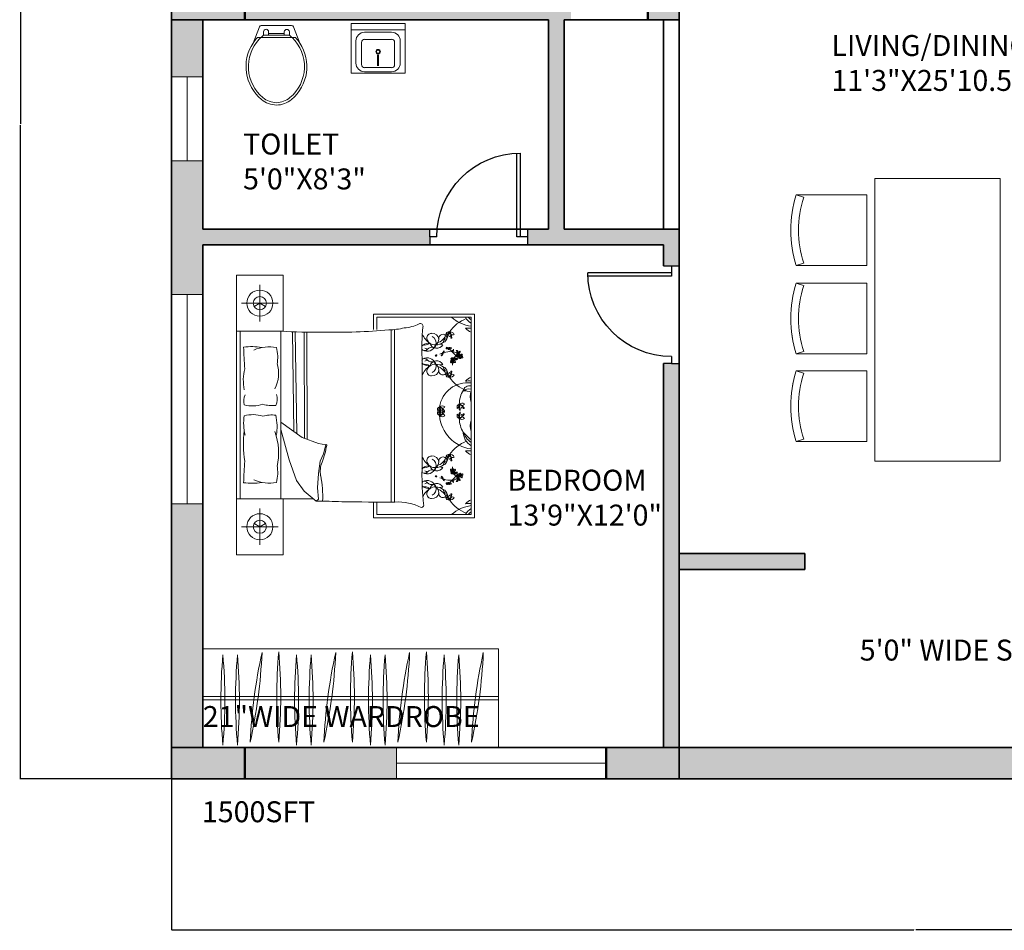
# Model space of a CAD drawing. Units: inches. Extents: x -28 to 485, y -861 to 54.
# Tile 1 of 14: x -28 to 254, y -861 to -600. Entities that reach past the tile are written whole.
import ezdxf

# ---------------------------------------------------------------- set-up
doc = ezdxf.new("R2010")
doc.units = ezdxf.units.IN
doc.header["$MEASUREMENT"] = 0
for name, color, linetype, lineweight in [('A-ANNO-DIMS', 2, 'Continuous', 18), ('A-ANNO-TEXT', 7, 'Continuous', 18), ('A-AREA-IDEN', 7, 'Continuous', 18), ('A-COLS', 7, 'Continuous', 50), ('A-COLS-PATT', 8, 'Continuous', 13), ('A-DOOR', 3, 'Continuous', 25), ('A-FLOR-CASE', 8, 'Continuous', 18), ('A-FLOR-FIXT', 9, 'Continuous', 18), ('A-FURN', 8, 'Continuous', 13), ('A-GLAZ', 4, 'Continuous', 18), ('A-WALL', 7, 'Continuous', 35), ('A-WALL-PATT', 34, 'Continuous', 13)]:
    doc.layers.add(name, color=color, linetype=linetype, lineweight=lineweight)
doc.styles.get("Standard").update_dxf_attribs({"font": 'arial.ttf'})
doc.dimstyles.get("Standard").update_dxf_attribs({"dimtxt": 0.18, "dimasz": 0.18, "dimexe": 0.18, "dimexo": 0.0625, "dimgap": 0.09, "dimtad": 0, "dimtih": 1, "dimtoh": 1, "dimdec": 0, "dimzin": 0, "dimdsep": 46, "dimlunit": 3, "dimtxsty": 'Standard', "dimcen": 0.09, "dimadec": 0, "dimazin": 0, "dimtfac": 1, "dimtdec": 0, "dimtofl": 0, "dimtmove": 0, "dimatfit": 3, "dimfxl": 1, "dimtolj": 1, "dimtzin": 0, "dimarcsym": 0})

# ---------------------------------------------------------------- blocks, each defined once
blk = doc.blocks.new('М14 600х655')
for p, q in [((-655, 600), (-655, 0)), ((-655, 600), (-655, 0)), ((-655, 0), (-655, 600)), ((0, 600), (-655, 600)), ((0, 0), (0, 600)), ((0, 525), (-655, 525)), ((-165, 494), (-490, 494)), ((-596, 388), (-596, 121)), ((-528, 370), (-528, 103)), ((-165, 408), (-490, 408)), ((-127, 103), (-127, 370)), ((-59, 121), (-59, 388)), ((-334, 87), (-334, 220)), ((-321, 87), (-321, 220)), ((-655, 0), (-655, 0)), ((-655, 0), (-655, 0)), ((-655, 0), (0, 0)), ((-655, 0), (0, 0)), ((-490, 65), (-165, 65)), ((-490, 15), (-165, 15))]:
    blk.add_line(p, q)
for radius in [27.6, 19.3]:
    blk.add_circle((-327, 259), radius)
for centre, radius, start, end in [((-490, 388), 106, 90, 180), ((-165, 388), 106, 0, 90), ((-490, 370), 38.2, 90, 180), ((-165, 370), 38.2, 0, 90), ((-490, 121), 106, 180, 270), ((-165, 121), 106, 270, 0), ((-490, 103), 38.2, 180, 270), ((-165, 103), 38.2, 270, 0)]:
    blk.add_arc(centre, radius, start, end)
blk = doc.blocks.new('BED-DOUBLE-WITH-NIGHTSTANDS')
for p, q in [((0, 0), (0, 80.08)), ((6.67, 66.84), (6.67, 77.31)), ((11.91, 72.08), (1.44, 72.08)), ((39.26, 64.51), (39.26, 68.96)), ((39.26, 68.96), (68.11, 68.96)), ((40.19, 68.03), (40.19, 64.5)), ((67.18, 68.03), (40.19, 68.03)), ((67.18, 11.5), (67.18, 68.03)), ((68.11, 68.96), (68.11, 10.57)), ((1.03, 64.07), (1.03, 16.02)), ((12.66, 16.02), (12.66, 64.07)), ((15.98, 63.85), (16.38, 35.34)), ((16.8, 63.82), (17.22, 34.74)), ((19.33, 63.78), (19.45, 33.37)), ((20.15, 63.78), (20.27, 33.06)), ((44.25, 64.43), (44.25, 15.09)), ((45.25, 64.51), (45.25, 15.09)), ((59.06, 60.14), (58.15, 60.31)), ((53.12, 56.3), (53.12, 23.78)), ((59.06, 54.54), (58.15, 54.36)), ((12.66, 38.02), (18.76, 33.63)), ((15.04, 27.14), (12.66, 35.87)), ((18.76, 33.63), (23.47, 31.84)), ((23.47, 31.84), (25.57, 31.52)), ((25.57, 31.52), (24.92, 28.93)), ((24.92, 28.93), (23.95, 26.82)), ((17.14, 21.3), (15.04, 27.14)), ((23.95, 26.82), (23.47, 23.25)), ((23.47, 23.25), (23.14, 19.19)), ((59.06, 24.99), (58.15, 25.16)), ((19.41, 18.22), (17.14, 21.3)), ((22.82, 15.3), (19.41, 18.22)), ((23.14, 19.19), (23.47, 15.95)), ((59.06, 19.39), (58.15, 19.21)), ((0, 16.02), (21.98, 16.02)), ((23.47, 15.95), (22.82, 15.3)), ((39.26, 10.57), (39.26, 15.1)), ((40.19, 15.1), (40.19, 11.5)), ((6.67, 13.24), (6.67, 2.78)), ((40.19, 11.5), (67.18, 11.5)), ((68.11, 10.57), (39.26, 10.57)), ((11.91, 8.01), (1.44, 8.01))]:
    blk.add_line(p, q)
for points in [[(0, 64.07), (13.35, 64.07), (13.35, 80.08), (0, 80.08)], [(6.67, 72.08), (5.06, 71.14)], [(6.67, 72.08), (8.29, 71.14)], [(13.35, 16.02), (13.35, 0), (0, 0)], [(6.67, 8.01), (5.06, 8.94)], [(6.67, 8.01), (8.29, 8.94)]]:
    blk.add_lwpolyline(points)
for points in [[(43.62, 64.41, 0.056112), (48.03, 64.99, 0.095341), (52.27, 66.12)], [(2, 59.47, -0.074897), (7.23, 59.37, 0.472817)], [(7.52, 43.09, -0.14099), (2.18, 42.93, -0.235245)], [(7.52, 39.67, 0.14099), (2.18, 39.83, 0.235245)], [(2, 20.62, 0.074897), (7.23, 20.71, -0.472817)], [(30.15, 15.13, 0.001242), (45.35, 15.09, -0.127202), (52.92, 13.49)]]:
    blk.add_lwpolyline(points, format="xyb")
for centre, radius in [((6.67, 72.08), 3.74), ((6.67, 72.08), 1.87), ((64.11, 56.84), 0.204), ((61.96, 55.51), 0.204), ((61.96, 24.02), 0.204), ((64.11, 22.68), 0.204), ((6.67, 8.01), 3.74), ((6.67, 8.01), 1.87)]:
    blk.add_circle(centre, radius)
for centre, radius, start, end in [((68.59, 75.81), 10.46, 228.1144, 262.255), ((69.99, 70.57), 5.1, 209.8884, 236.5383), ((70.94, 72.4), 6.35, 223.5186, 233.6964), ((52.68, 65.51), 0.73, 336.5219, 123.8264), ((131.01, 58.75), 77.93, 175.2402, 181.8035), ((69.62, 57.92), 10.46, 111.4092, 145.6135), ((68.81, 67.71), 4.25, 221.0454, 247.4453), ((66.52, 79.36), 14.47, 266.3481, 272.5919), ((22.44, 207.63), 143.9, 266.1, 270.9282), ((27.68, 251.44), 187.71, 269.1145, 274.8735), ((58.76, 65.61), 6.06, 203.6453, 236.3329), ((55.85, 62.08), 1.35, 88.9462, 185.5144), ((56.04, 61.53), 1.91, 7.1143, 95.0551), ((55.32, 60.77), 1.86, 338.5779, 68.4181), ((56.48, 64.35), 3.78, 288.2955, 328.7386), ((59.12, 61.97), 1.2, 19.1312, 189.736), ((58.76, 62.26), 1.5, 285.6955, 4.031), ((60.43, 62.21), 0.737, 126.7319, 206.0245), ((60.79, 62.99), 0.867, 76.272, 177.0484), ((59.47, 64.76), 1.79, 284.7031, 328.6173), ((61.96, 62.49), 1.65, 125.7657, 194.5347), ((53.85, 65.41), 7.32, 332.8176, 347.4827), ((61.24, 62.69), 1.16, 20.9613, 102.2885), ((61.86, 63.85), 0.873, 181.7131, 301.5367), ((59, 62.09), 2.64, 2.0648, 41.1598), ((60.59, 63.07), 0.856, 316.2238, 62.3173), ((61.09, 62.57), 0.0682, 20.2667, 316.2271), ((61.51, 62.18), 0.13, 168.5166, 2.0648), ((61.45, 62.19), 0.0631, 52.0591, 168.5166), ((-760.15, 15.33), 763.42, 2.85022, 3.31479), ((9.33, 49.26), 10.32, 78.2417, 114.8684), ((1.06, 56.61), 10.73, 348.9631, 14.8961), ((54, 59.28), 0.964, 127.675, 162.5814), ((53.71, 63.39), 3.32, 259.249, 301.1782), ((54.57, 60.82), 2.55, 240.8249, 340.7178), ((55.15, 57.49), 3.09, 85.2696, 124.215), ((56.85, 62.5), 2.41, 193.079, 274.7067), ((55.94, 57.8), 1.64, 74.8529, 138.4347), ((57.33, 61.13), 1.99, 196.8663, 330.0915), ((56.5, 59.87), 0.497, 254.8529, 12.6959), ((55.15, 57.49), 3.09, 53.6555, 57.2989), ((55.62, 61.86), 2.33, 305.9599, 357.6409), ((56.78, 64.39), 4.3, 273.4924, 303.7117), ((60.76, 60.64), 1.6, 128.4175, 173.8338), ((60.19, 59.12), 0.158, 125.0752, 284.7644), ((60.43, 59.18), 0.34, 127.3642, 168.4363), ((60.17, 59.45), 0.49, 277.4968, 341.2737), ((60.56, 59.22), 0.195, 88.1325, 178.8919), ((60.95, 59.02), 0.422, 136.3462, 189.6513), ((60.75, 59.46), 0.204, 183.2768, 356.7232), ((61.39, 59.1), 0.668, 164.2829, 186.9148), ((60.6, 59.09), 0.334, 312.3208, 40.2111), ((61.31, 59.47), 0.474, 201.6382, 274.947), ((60.68, 58.82), 0.619, 42.3896, 66.5724), ((61.13, 59.18), 0.337, 10.9597, 52.2379), ((61.33, 59.15), 0.156, 274.947, 37.5263), ((54, 59.28), 0.964, 196.6343, 225.5483), ((53.81, 59.69), 1.2, 246.1646, 318.4347), ((55.03, 61.2), 2.3, 240.0851, 262.564), ((57.16, 57.12), 0.251, 169.5864, 349.5616), ((57.25, 57.11), 0.154, 349.5616, 167.2949), ((61.28, 51.56), 6.63, 110.1059, 116.9968), ((59.06, 57.02), 0.42, 129.5056, 182.6421), ((57.85, 58), 1.27, 308.4388, 328.836), ((57.63, 59.02), 2.26, 296.5064, 305.3102), ((57.61, 57.86), 1.29, 336.3901, 344.4871), ((59.01, 57.53), 0.163, 83.9457, 185.6216), ((58.36, 57.69), 0.671, 328.836, 0.8141), ((58.71, 57.49), 0.384, 306.5232, 32.4668), ((59.16, 57.79), 0.163, 112.5583, 214.2343), ((59.06, 58.08), 0.384, 265.7131, 351.6568), ((58.72, 58.29), 0.671, 297.3659, 329.344), ((58.21, 58.87), 1.29, 313.6929, 321.7899), ((59.64, 57.99), 0.42, 115.5379, 168.6744), ((58.21, 58.6), 1.27, 329.344, 349.7412), ((61.28, 51.56), 6.63, 86.1723, 106.4158), ((57.2, 58.31), 2.26, 352.8698, 1.6736), ((60.71, 58.98), 0.176, 189.6513, 312.3208), ((66.93, 63.72), 7.6, 217.9541, 226.8459), ((61.66, 57.07), 0.93, 253.6301, 325.4631), ((61.92, 55.78), 0.658, 82.0748, 142.6895), ((61.86, 58.27), 0.163, 112.5583, 214.2343), ((61.75, 58.56), 0.384, 265.7131, 351.6568), ((61.42, 58.77), 0.671, 297.3659, 329.344), ((61.45, 54.86), 3.33, 60.7959, 85.244), ((54.37, 50.07), 10.94, 37.8256, 47.7588), ((60.91, 59.35), 1.29, 313.6929, 321.7899), ((61.87, 56.57), 0.565, 273.8774, 357.1501), ((62.33, 58.47), 0.42, 115.5379, 168.6744), ((60.9, 59.07), 1.27, 329.344, 349.7412), ((62.09, 56.97), 0.547, 262.0748, 308.2393), ((59.89, 58.78), 2.26, 352.8698, 1.6736), ((62.87, 56.86), 0.547, 215.1128, 261.2773), ((63.31, 56.83), 0.93, 197.889, 269.722), ((65.87, 54.52), 3.99, 130.182, 149.456), ((63.07, 58.33), 0.228, 33.0979, 123.1364), ((58.05, 55.12), 5.96, 31.1156, 34.8118), ((62.74, 57.94), 0.617, 2.3172, 70.5201), ((63.67, 56.79), 0.658, 139.3812, 199.9959), ((62.44, 57.27), 0.93, 310.9365, 22.7695), ((62.87, 57.22), 0.675, 285.6484, 332.2957), ((63.25, 57.78), 0.178, 135.7354, 318.1297), ((62.95, 58.07), 0.236, 315.7354, 31.1156), ((62.75, 57.57), 0.547, 319.3812, 5.5456), ((63.38, 57.79), 0.178, 68.2452, 250.6395), ((62.97, 58), 0.531, 352.6008, 57.1845), ((64.87, 54.44), 3.55, 111.7087, 116.2181), ((61.45, 54.86), 3.33, 47.5083, 55.9967), ((63.48, 58.12), 0.531, 252.8042, 349.6943), ((62.97, 57.17), 0.565, 331.1838, 51.6792), ((63.55, 56.5), 0.158, 125.0752, 284.7644), ((63.53, 58.17), 0.236, 248.2452, 323.6254), ((63.8, 56.56), 0.34, 93.635, 168.4363), ((63.33, 58.31), 0.617, 291.7087, 3.0299), ((63.75, 57.1), 0.2, 138.2946, 276.2474), ((63.53, 56.83), 0.49, 277.4968, 341.2737), ((63.83, 57.07), 0.278, 358.5719, 143.8954), ((58.93, 61.56), 5.96, 323.6254, 327.3216), ((63.92, 56.61), 0.195, 88.1325, 178.8919), ((63.99, 57.29), 0.281, 208.8493, 269.9355), ((63.75, 57.22), 0.321, 274.2123, 318.1587), ((64.31, 56.4), 0.422, 136.3462, 189.6513), ((63.81, 58.16), 0.228, 325.6077, 55.6462), ((64.75, 56.48), 0.668, 164.2829, 186.9148), ((64.73, 56.9), 0.643, 121.9501, 165.2442), ((63.96, 56.47), 0.334, 312.3208, 40.2111), ((64.67, 56.85), 0.474, 201.6382, 274.947), ((64.28, 57.14), 0.135, 262.868, 7.094), ((64.04, 56.2), 0.619, 42.3896, 66.5724), ((64.27, 57.26), 0.403, 278.5614, 22.5914), ((64.49, 56.56), 0.337, 10.9597, 118.7804), ((64.49, 57.27), 0.202, 44.3732, 121.9501), ((64.7, 56.53), 0.156, 274.947, 37.5263), ((1.85, 51.98), 10.19, 333.8761, 16.1746), ((54, 55.39), 0.964, 134.4517, 156.7144), ((54, 55.39), 0.964, 203.2856, 232.325), ((53.71, 51.28), 3.32, 58.8218, 100.2867), ((58.76, 49.06), 6.06, 123.6671, 158.5059), ((54.57, 53.85), 2.55, 19.2822, 119.1751), ((53.81, 54.99), 1.2, 41.5653, 113.8354), ((55.15, 57.18), 3.09, 235.785, 274.7304), ((55.03, 53.47), 2.3, 97.436, 119.9149), ((56.85, 52.18), 2.41, 85.2933, 166.921), ((55.94, 56.87), 1.64, 221.5653, 285.1471), ((57.33, 53.55), 1.99, 29.9085, 163.1337), ((55.32, 53.9), 1.86, 291.5819, 21.4221), ((56.5, 54.81), 0.497, 347.3041, 105.1471), ((55.15, 57.18), 3.09, 302.7011, 306.3445), ((55.62, 52.81), 2.33, 2.3591, 54.0401), ((56.78, 50.29), 4.3, 56.2883, 86.5076), ((56.48, 50.32), 3.78, 31.2614, 71.7045), ((60.76, 54.03), 1.6, 186.1662, 231.5825), ((58.76, 52.42), 1.5, 355.969, 74.3045), ((61.4, 55.17), 0.158, 125.0752, 284.7644), ((61.65, 55.23), 0.34, 93.635, 168.4363), ((61.85, 56.68), 0.675, 228.342, 274.9894), ((61.6, 55.76), 0.2, 138.2946, 276.2474), ((61.38, 55.5), 0.49, 277.4968, 341.2737), ((61.68, 55.73), 0.278, 358.5719, 143.8954), ((61.77, 55.27), 0.195, 88.1325, 178.8919), ((61.84, 55.95), 0.281, 208.8493, 269.9355), ((61.6, 55.89), 0.321, 274.2123, 318.1587), ((62.16, 55.06), 0.422, 136.3462, 189.6513), ((61.92, 55.02), 0.176, 189.6513, 312.3208), ((65.87, 54.52), 3.99, 175.2415, 182.8929), ((62.6, 55.14), 0.668, 164.2829, 186.9148), ((62.58, 55.56), 0.643, 121.9501, 165.2442), ((61.81, 55.14), 0.334, 312.3208, 40.2111), ((62.52, 55.52), 0.474, 201.6382, 274.947), ((62.13, 55.81), 0.135, 262.868, 7.094), ((61.89, 54.87), 0.619, 42.3896, 66.5724), ((62.12, 55.92), 0.403, 278.5614, 22.5914), ((62.34, 55.23), 0.337, 10.9597, 118.7804), ((65.87, 54.52), 3.99, 156.1523, 156.9499), ((62.34, 55.94), 0.202, 44.3732, 121.9501), ((62.97, 56.41), 0.565, 181.4625, 249.4747), ((62.55, 55.2), 0.156, 274.947, 37.5263), ((63.02, 56.51), 0.675, 248.3627, 295.0101), ((62.69, 55.67), 0.658, 20.6625, 81.2773), ((64.07, 56.36), 0.176, 189.6513, 312.3208), ((16.01, 49.96), 14.08, 166.3427, 191.1841), ((55.85, 52.59), 1.35, 174.4856, 271.0538), ((56.04, 53.15), 1.91, 264.9449, 352.8857), ((59.12, 52.71), 1.2, 170.264, 340.8688), ((60.43, 52.46), 0.737, 153.9755, 233.2681), ((60.79, 51.69), 0.867, 182.9516, 283.728), ((59.47, 49.92), 1.79, 31.3827, 75.2969), ((61.96, 52.19), 1.65, 165.4653, 234.2343), ((53.85, 49.26), 7.32, 12.5173, 27.1824), ((59, 52.59), 2.64, 318.8402, 357.9352), ((60.59, 51.6), 0.856, 297.6827, 43.7762), ((61.86, 50.82), 0.873, 58.4633, 178.2869), ((61.24, 51.98), 1.16, 257.7115, 339.0387), ((69.62, 56.75), 10.46, 214.3865, 248.5908), ((61.13, 52.12), 0.113, 43.7762, 339.7183), ((61.51, 52.5), 0.13, 357.9352, 191.4834), ((61.45, 52.48), 0.0631, 191.4834, 307.9409), ((68.81, 46.96), 4.25, 112.5547, 138.9546), ((66.17, 41.19), 8.09, 82.8636, 171.8197), ((66.74, 46.53), 1.88, 76.3898, 169.0739), ((66.52, 35.31), 14.47, 87.4081, 93.6519), ((5.99, 44.03), 3.96, 153.3437, 196.1026), ((7.37, 44.56), 4.25, 335.0183, 18.5407), ((74.19, 42.33), 10.46, 152.5854, 175.5377), ((66.48, 45.12), 2.37, 72.8609, 131.9049), ((65.43, 42.24), 4.68, 68.117, 96.6195), ((72.68, 45.26), 5.75, 162.9798, 196.4569), ((10.2, 52.53), 9.81, 254.1707, 275.9871), ((58.4, 41.51), 0.867, 106.1963, 206.9726), ((56.38, 42.39), 1.79, 314.6273, 358.5415), ((59.67, 41.66), 1.65, 155.6899, 224.4589), ((58.94, 41.49), 1.16, 50.8855, 132.2127), ((58.91, 42.8), 0.873, 211.6373, 331.4609), ((58.2, 41.49), 0.856, 346.148, 92.2415), ((57.3, 39.84), 2.64, 31.989, 71.0841), ((51.18, 40.16), 7.32, 2.7418, 17.407), ((64.01, 42.31), 0.867, 106.1963, 206.9726), ((61.98, 43.19), 1.79, 314.6273, 358.5415), ((65.27, 42.46), 1.65, 155.6899, 224.4589), ((64.54, 42.29), 1.16, 50.8855, 132.2127), ((64.51, 43.6), 0.873, 211.6373, 331.4609), ((63.8, 42.29), 0.856, 346.148, 92.2415), ((62.91, 40.64), 2.64, 31.989, 71.0841), ((56.78, 40.96), 7.32, 2.7418, 17.407), ((75.64, 42.98), 8.5, 174.3643, 175.6213), ((81.47, 38.5), 15.2, 160.0972, 160.2783), ((16.3, 37.72), 14.27, 171.5249, 193.96), ((10.2, 30.23), 9.81, 84.0129, 105.8293), ((-2.51, 36.66), 14.12, 349.8617, 13.6238), ((58.4, 40.68), 0.867, 153.0274, 253.8037), ((56.38, 39.81), 1.79, 1.4585, 45.3727), ((59.67, 40.53), 1.65, 135.5411, 204.3101), ((51.18, 42.04), 7.32, 342.593, 357.2582), ((57.3, 42.35), 2.64, 288.9159, 328.011), ((58.2, 40.71), 0.856, 267.7585, 13.852), ((58.91, 39.39), 0.873, 28.5391, 148.3627), ((58.94, 40.71), 1.16, 227.7873, 309.1145), ((68.59, 40.66), 10.46, 184.4623, 262.255), ((58.87, 41.3), 0.0682, 50.1909, 346.0209), ((58.92, 40.88), 0.113, 13.852, 309.9245), ((59.44, 41.17), 0.13, 198.4408, 31.989), ((59.37, 41.15), 0.0631, 81.9833, 198.4408), ((59.44, 41.02), 0.13, 328.011, 161.5592), ((59.37, 41.04), 0.0631, 161.5592, 278.0167), ((64.01, 39.88), 0.867, 153.0274, 253.8037), ((61.98, 39.01), 1.79, 1.4585, 45.3727), ((65.27, 39.73), 1.65, 135.5411, 204.3101), ((56.78, 41.24), 7.32, 342.593, 357.2582), ((62.91, 41.55), 2.64, 288.9159, 328.011), ((63.8, 39.91), 0.856, 267.7585, 13.852), ((64.52, 40.08), 0.113, 13.852, 309.9245), ((64.47, 42.1), 0.0682, 50.1909, 346.0209), ((64.98, 41.95), 0.0631, 81.9833, 198.4408), ((64.98, 40.24), 0.0631, 161.5592, 278.0167), ((65.04, 41.98), 0.13, 198.4408, 31.989), ((65.04, 40.22), 0.13, 328.011, 161.5592), ((64.51, 38.59), 0.873, 28.5391, 148.3627), ((64.54, 39.91), 1.16, 227.7873, 309.1145), ((74.19, 39.86), 10.46, 184.4623, 207.4146), ((72.68, 36.94), 5.75, 163.5431, 197.0202), ((75.64, 39.22), 8.5, 184.3787, 185.6357), ((81.47, 43.7), 15.2, 199.7217, 199.9028), ((30.98, 31.59), 29.04, 172.2196, 189.497), ((-6.57, 29.12), 18.61, 348.0397, 19.2615), ((69.99, 35.42), 5.1, 181.272, 236.5383), ((72.72, 40.59), 9.45, 214.0123, 234.053), ((70.94, 37.25), 6.35, 197.8504, 233.6964), ((-4.69, 37.08), 31.06, 340.1194, 349.3383), ((25.64, 31.34), 0.193, 358.8623, 109.7536), ((69.62, 22.77), 10.46, 111.4092, 145.6135), ((58.76, 30.46), 6.06, 201.4941, 236.3329), ((55.85, 26.93), 1.35, 88.9462, 185.5144), ((56.04, 26.38), 1.91, 7.1143, 95.0551), ((60.79, 27.84), 0.867, 76.272, 177.0484), ((59.47, 29.61), 1.79, 284.7031, 328.6173), ((61.96, 27.34), 1.65, 125.7657, 194.5347), ((53.85, 30.27), 7.32, 332.8176, 347.4827), ((61.24, 27.55), 1.16, 20.9613, 102.2885), ((60.59, 27.92), 0.856, 316.2238, 62.3173), ((59, 26.94), 2.64, 2.0648, 41.1598), ((61.86, 28.71), 0.873, 181.7131, 301.5367), ((66.52, 44.21), 14.47, 266.3481, 272.5919), ((68.81, 32.56), 4.25, 221.0454, 247.4453), ((-760.15, 64.76), 763.42, 356.68521, 357.14978), ((1.06, 23.47), 10.73, 345.1039, 11.0369), ((30.48, 23.89), 6.52, 156.2616, 191.3392), ((53.71, 28.24), 3.32, 259.7133, 301.1782), ((55.15, 22.34), 3.09, 85.2696, 124.215), ((56.85, 27.35), 2.41, 193.079, 274.7067), ((57.33, 25.98), 1.99, 196.8663, 330.0915), ((55.32, 25.63), 1.86, 338.5779, 68.4181), ((55.62, 26.71), 2.33, 305.9599, 357.6409), ((56.78, 29.24), 4.3, 273.4924, 303.7117), ((56.48, 29.2), 3.78, 288.2955, 328.7386), ((59.12, 26.82), 1.2, 19.1312, 189.736), ((58.76, 27.11), 1.5, 285.6955, 4.031), ((60.76, 25.49), 1.6, 128.4175, 173.8338), ((60.43, 27.07), 0.737, 126.7319, 206.0245), ((61.09, 27.42), 0.0682, 20.2667, 316.2271), ((61.51, 27.03), 0.13, 168.5166, 2.0648), ((61.45, 27.04), 0.0631, 52.0591, 168.5166), ((-5.54, 16.67), 30.23, 357.4519, 11.3392), ((136.48, 22.83), 83.37, 179.3433, 185.6887), ((54, 24.13), 0.964, 127.675, 156.7144), ((54, 24.13), 0.964, 203.229, 225.5483), ((54.57, 25.67), 2.55, 240.8249, 340.7178), ((53.81, 24.54), 1.2, 246.1646, 318.4347), ((55.03, 26.06), 2.3, 240.0851, 262.564), ((55.94, 22.65), 1.64, 74.8529, 138.4347), ((56.5, 24.72), 0.497, 254.8529, 12.6959), ((55.15, 22.34), 3.09, 53.6555, 57.2989), ((57.16, 22.4), 0.251, 10.4384, 190.4136), ((61.4, 24.36), 0.158, 75.2356, 234.9248), ((61.65, 24.3), 0.34, 191.5637, 266.365), ((61.6, 23.76), 0.2, 83.7526, 221.7054), ((61.85, 22.84), 0.675, 85.0106, 131.658), ((61.66, 22.46), 0.93, 34.5369, 106.3699), ((61.92, 23.75), 0.658, 217.3105, 277.9252), ((61.38, 24.03), 0.49, 18.7263, 82.5032), ((61.68, 23.79), 0.278, 216.1046, 1.4281), ((61.77, 24.25), 0.195, 181.1081, 271.8675), ((61.84, 23.57), 0.281, 90.0645, 151.1507), ((61.6, 23.64), 0.321, 41.8413, 85.7877), ((54.37, 29.45), 10.94, 312.2412, 322.1744), ((61.92, 24.5), 0.176, 47.6792, 170.3487), ((62.16, 24.46), 0.422, 170.3487, 223.6538), ((65.87, 25.01), 3.99, 177.1071, 184.7585), ((61.87, 22.95), 0.565, 2.8499, 86.1226), ((62.6, 24.38), 0.668, 173.0852, 195.7171), ((62.58, 23.96), 0.643, 194.7558, 238.0499), ((62.09, 22.55), 0.547, 51.7607, 97.9252), ((61.81, 24.39), 0.334, 319.7889, 47.6792), ((62.52, 24.01), 0.474, 85.053, 158.3618), ((62.13, 23.71), 0.135, 352.906, 97.132), ((61.89, 24.66), 0.619, 293.4276, 317.6104), ((62.34, 24.29), 0.337, 241.2196, 349.0403), ((62.12, 23.6), 0.403, 337.4086, 81.4386), ((65.87, 25.01), 3.99, 203.0501, 203.8477), ((62.34, 23.59), 0.202, 238.0499, 315.6268), ((62.97, 23.11), 0.565, 110.5253, 178.5375), ((63.31, 22.7), 0.93, 90.278, 162.111), ((62.87, 22.67), 0.547, 98.7227, 144.8872), ((65.87, 25.01), 3.99, 210.544, 229.818), ((62.55, 24.33), 0.156, 322.4737, 85.053), ((63.02, 23.01), 0.675, 64.9899, 111.6373), ((62.69, 23.86), 0.658, 278.7227, 339.3375), ((63.67, 22.74), 0.658, 160.0041, 220.6188), ((62.44, 22.26), 0.93, 337.2305, 49.0635), ((62.87, 22.31), 0.675, 27.7043, 74.3516), ((62.97, 22.35), 0.565, 308.3208, 28.8162), ((63.55, 23.03), 0.158, 75.2356, 234.9248), ((63.8, 22.96), 0.34, 191.5637, 266.365), ((63.75, 22.43), 0.2, 83.7526, 221.7054), ((63.53, 22.69), 0.49, 18.7263, 82.5032), ((63.92, 22.92), 0.195, 181.1081, 271.8675), ((63.75, 22.31), 0.321, 41.8413, 85.7877), ((64.07, 23.17), 0.176, 47.6792, 170.3487), ((64.31, 23.13), 0.422, 170.3487, 223.6538), ((64.75, 23.05), 0.668, 173.0852, 195.7171), ((63.96, 23.05), 0.334, 319.7889, 47.6792), ((64.67, 22.68), 0.474, 85.053, 158.3618), ((64.04, 23.32), 0.619, 293.4276, 317.6104), ((64.49, 22.96), 0.337, 241.2196, 349.0403), ((64.27, 22.27), 0.403, 337.4086, 81.4386), ((64.7, 22.99), 0.156, 322.4737, 85.053), ((9.33, 30.82), 10.32, 245.1316, 281.7583), ((54, 20.25), 0.964, 134.4517, 153.558), ((54, 20.25), 0.964, 210.0293, 232.325), ((54.57, 18.71), 2.55, 19.2822, 119.1751), ((53.81, 19.84), 1.2, 41.5653, 113.8354), ((55.03, 18.32), 2.3, 97.436, 119.9149), ((55.94, 21.72), 1.64, 221.5653, 285.1471), ((57.33, 18.4), 1.99, 29.9085, 163.1337), ((56.5, 19.66), 0.497, 347.3041, 105.1471), ((57.25, 22.42), 0.154, 192.7051, 10.4384), ((61.28, 27.97), 6.63, 243.0032, 249.8941), ((57.85, 21.53), 1.27, 31.164, 51.5612), ((59.06, 22.5), 0.42, 177.3579, 230.4944), ((57.63, 20.5), 2.26, 54.6898, 63.4936), ((57.61, 21.66), 1.29, 15.5129, 23.6099), ((59.01, 21.99), 0.163, 174.3784, 276.0543), ((58.71, 22.03), 0.384, 327.5332, 53.4768), ((58.36, 21.84), 0.671, 359.1859, 31.164), ((59.16, 21.74), 0.163, 145.7657, 247.4417), ((59.06, 21.45), 0.384, 8.3432, 94.2869), ((58.72, 21.23), 0.671, 30.656, 62.6341), ((58.21, 20.66), 1.29, 38.2101, 46.3071), ((59.64, 21.53), 0.42, 191.3256, 244.4621), ((58.21, 20.93), 1.27, 10.2588, 30.656), ((61.28, 27.97), 6.63, 253.5842, 273.8277), ((57.2, 21.22), 2.26, 358.3264, 7.1302), ((60.19, 20.41), 0.158, 75.2356, 234.9248), ((60.43, 20.35), 0.34, 191.5637, 232.6358), ((60.17, 20.07), 0.49, 18.7263, 82.5032), ((60.56, 20.3), 0.195, 181.1081, 271.8675), ((60.71, 20.55), 0.176, 47.6792, 170.3487), ((60.95, 20.51), 0.422, 170.3487, 223.6538), ((60.75, 20.06), 0.204, 3.2768, 176.7232), ((61.39, 20.43), 0.668, 173.0852, 195.7171), ((60.6, 20.43), 0.334, 319.7889, 47.6792), ((61.31, 20.06), 0.474, 85.053, 158.3618), ((60.68, 20.7), 0.619, 293.4276, 317.6104), ((66.93, 15.8), 7.6, 133.1541, 142.0459), ((61.13, 20.34), 0.337, 307.7621, 349.0403), ((61.33, 20.37), 0.156, 322.4737, 85.053), ((61.86, 21.26), 0.163, 145.7657, 247.4417), ((61.45, 24.67), 3.33, 274.756, 299.2041), ((61.75, 20.97), 0.384, 8.3432, 94.2869), ((61.42, 20.76), 0.671, 30.656, 62.6341), ((60.91, 20.18), 1.29, 38.2101, 46.3071), ((62.33, 21.06), 0.42, 191.3256, 244.4621), ((60.9, 20.45), 1.27, 10.2588, 30.656), ((59.89, 20.74), 2.26, 358.3264, 7.1302), ((62.74, 21.59), 0.617, 289.4799, 357.6828), ((58.05, 24.41), 5.96, 325.1882, 328.8844), ((63.07, 21.2), 0.228, 236.8636, 326.9021), ((63.25, 21.74), 0.178, 41.8703, 224.2646), ((62.95, 21.45), 0.236, 328.8844, 44.2646), ((62.75, 21.95), 0.547, 354.4544, 40.6188), ((63.38, 21.74), 0.178, 109.3605, 291.7548), ((62.97, 21.52), 0.531, 302.8155, 7.3992), ((64.87, 25.09), 3.55, 243.7819, 248.2913), ((61.45, 24.67), 3.33, 304.0033, 312.4917), ((63.48, 21.4), 0.531, 10.3057, 107.1958), ((63.53, 21.36), 0.236, 36.3746, 111.7548), ((63.33, 21.21), 0.617, 356.9701, 68.2913), ((63.83, 22.46), 0.278, 216.1046, 1.4281), ((58.93, 17.96), 5.96, 32.6784, 36.3746), ((63.99, 22.24), 0.281, 90.0645, 151.1507), ((63.81, 21.37), 0.228, 304.3538, 34.3923), ((64.73, 22.63), 0.643, 194.7558, 238.0499), ((64.28, 22.38), 0.135, 352.906, 97.132), ((64.49, 22.25), 0.202, 238.0499, 315.6268), ((53.71, 16.14), 3.32, 58.8218, 99.1554), ((58.76, 13.91), 6.06, 123.6671, 153.2997), ((55.15, 22.04), 3.09, 235.785, 274.7304), ((56.85, 17.03), 2.41, 85.2933, 166.921), ((55.85, 17.44), 1.35, 174.4856, 271.0538), ((56.04, 18), 1.91, 264.9449, 352.8857), ((55.32, 18.75), 1.86, 291.5819, 21.4221), ((55.15, 22.04), 3.09, 302.7011, 306.3445), ((55.62, 17.67), 2.33, 2.3591, 54.0401), ((56.78, 15.14), 4.3, 56.2883, 86.5076), ((56.48, 15.18), 3.78, 31.2614, 71.7045), ((59.12, 17.56), 1.2, 170.264, 340.8688), ((58.76, 17.27), 1.5, 355.969, 74.3045), ((60.76, 18.89), 1.6, 186.1662, 231.5825), ((60.43, 17.31), 0.737, 153.9755, 233.2681), ((61.96, 17.04), 1.65, 165.4653, 234.2343), ((53.85, 14.11), 7.32, 12.5173, 27.1824), ((59, 17.44), 2.64, 318.8402, 357.9352), ((60.59, 16.46), 0.856, 297.6827, 43.7762), ((61.13, 16.97), 0.113, 43.7762, 339.7183), ((61.51, 17.35), 0.13, 357.9352, 191.4834), ((61.45, 17.33), 0.0631, 191.4834, 307.9409), ((24.81, -58.13), 73.46, 85.8294, 91.553), ((52.87, 14.23), 0.739, 273.98, 27.3412), ((59.47, 14.77), 1.79, 31.3827, 75.2969), ((60.79, 16.54), 0.867, 182.9516, 283.728), ((61.86, 15.67), 0.873, 58.4633, 178.2869), ((61.24, 16.83), 1.16, 257.7115, 339.0387), ((69.62, 21.6), 10.46, 214.3865, 248.5908), ((68.81, 11.81), 4.25, 112.5547, 138.9546), ((66.52, 0.17), 14.47, 87.4081, 93.6519), ((68.59, 3.71), 10.46, 97.745, 131.8856), ((69.99, 8.96), 5.1, 123.4617, 150.1116), ((70.94, 7.13), 6.35, 126.3036, 136.4814)]:
    blk.add_arc(centre, radius, start, end)
blk = doc.blocks.new('WARDROBE-HANGING')
for p, q in [((84.7, 28.23), (0, 28.23)), ((0, 28.23), (0, 0)), ((84.7, 28.23), (84.7, 0)), ((84.7, 14.59), (0, 14.59)), ((84.7, 13.65), (0, 13.65)), ((84.7, 0), (0, 0))]:
    blk.add_line(p, q)
for centre, start, end in [((153.74, 13.55), 175.0028, 184.9972), ((-142.25, 13.55), 355.0028, 4.9972), ((157.93, 13.55), 175.0028, 184.9972), ((-138.07, 13.55), 355.0028, 4.9972), ((-131.46, 33.65), 347.508, 357.5023), ((162.01, -4.96), 167.508, 177.5023), ((169.76, 14.46), 175.0028, 184.9972), ((-126.23, 14.46), 355.0028, 4.9972), ((174.85, 13.55), 175.0028, 184.9972), ((-121.15, 13.55), 355.0028, 4.9972), ((179.03, 13.55), 175.0028, 184.9972), ((-116.97, 13.55), 355.0028, 4.9972), ((-110.36, 33.65), 347.508, 357.5023), ((183.11, -4.96), 167.508, 177.5023), ((190.86, 14.46), 175.0028, 184.9972), ((-105.13, 14.46), 355.0028, 4.9972), ((196.03, 13.55), 175.0028, 184.9972), ((-99.97, 13.55), 355.0028, 4.9972), ((200.21, 13.55), 175.0028, 184.9972), ((-95.78, 13.55), 355.0028, 4.9972), ((204.29, -4.96), 167.508, 177.5023), ((-89.17, 33.65), 347.508, 357.5023), ((212.05, 14.46), 175.0028, 184.9972), ((-83.95, 14.46), 355.0028, 4.9972), ((217.13, 13.55), 175.0028, 184.9972), ((-78.86, 13.55), 355.0028, 4.9972), ((221.31, 13.55), 175.0028, 184.9972), ((-74.68, 13.55), 355.0028, 4.9972), ((225.4, -4.96), 167.508, 177.5023), ((-68.07, 33.65), 347.508, 357.5023)]:
    blk.add_arc(centre, 148.56, start, end)
blk = doc.blocks.new('WC-FLOOR-MOUNTED')
for p, q in [((3.27, 19.35), (4.23, 19.35)), ((4.23, 19.35), (8.71, 19.35)), ((13.2, 19.35), (8.71, 19.35)), ((13.2, 19.35), (14.16, 19.35))]:
    blk.add_line(p, q)
for points in [[(8.71, 22.81), (4.36, 22.81, 0.31031), (3.82, 22.44), (2.03, 17.79, 0.209071)], [(8.71, 22.81), (13.07, 22.81, -0.31031), (13.6, 22.44), (15.39, 17.79, -0.209071)], [(5.01, 20.04, 0.022712), (4.23, 19.35, 0.162618)], [(5.01, 20.04), (5.01, 21, -1), (6.47, 21), (6.47, 20.5)], [(8.71, 20.04), (5.01, 20.04, 0.022712)], [(8.71, 20.04), (12.41, 20.04, -0.476108)], [(12.41, 20.04), (12.41, 21, 1), (10.96, 21), (10.96, 20.5)], [(12.41, 20.04, -0.022712), (13.2, 19.35, -0.162618)], [(2.03, 17.79, 0.383919), (4.43, 1.64, 0.163732), (8.71, 0, 0.359733)], [(3.77, 18.89, 0.431639), (4.86, 2.17, 0.162618), (8.71, 0.68, 0.470877)], [(3.27, 19.35, 0.040937), (2.03, 17.79, 0.163732)], [(4.23, 19.35, 0.014165), (3.77, 18.89, 0.162618)], [(13.2, 19.35, -0.448546), (12.57, 2.17, -0.162618), (8.71, 0.68, -0.470877)], [(15.39, 17.79, -0.383919), (13, 1.64, -0.163732), (8.71, 0, -0.359733)], [(14.16, 19.35, -0.040937), (15.39, 17.79, -0.163732)]]:
    blk.add_lwpolyline(points, format="xyb")
for points in [[(10.96, 20.5), (6.47, 20.5)], [(6.47, 20.5), (6.47, 20.04)], [(10.96, 20.5), (10.96, 20.04)]]:
    blk.add_lwpolyline(points)
blk = doc.blocks.new('CHAIR-DINING')
for p, q in [((20.22, 20.23), (18.08, 19.55)), ((20.22, 0), (18.08, 0.68))]:
    blk.add_line(p, q)
blk.add_lwpolyline([(20.23, 0), (0, 0), (0, 20.23), (20.23, 20.23, -0.153703), (20.23, 0)], format="xyb")
for radius in [33.37, 31.13]:
    blk.add_arc((-11.59, 10.12), radius, 342.3544, 17.6456)
blk = doc.blocks.new('TABLE-DINING-RECT')
blk.add_lwpolyline([(0, 80.93), (35.97, 80.93), (35.97, 0), (0, 0)], close=True)
blk = doc.blocks.new('DOOR-SWING-24')
for p, q in [((2, 2.25), (2, 26.25)), ((3, 2.25), (3, 26.25)), ((0, 4.5), (0, 0)), ((28, 2.25), (28, 4.5)), ((0, 2.25), (2, 2.25)), ((2, 2.25), (3, 2.25)), ((26, 2.25), (28, 2.25)), ((28, 2.25), (28, 0))]:
    blk.add_line(p, q)
blk.add_arc((2, 2.25), 24, 0, 90)
blk = doc.blocks.new('WINDOW-60IN')
for p, q in [((0, 60), (0, 0)), ((9, 60), (0, 60)), ((4.5, 60), (4.5, 0)), ((9, 0), (9, 60)), ((0, 0), (9, 0))]:
    blk.add_line(p, q)
blk = doc.blocks.new('WINDOW-24IN')
for p, q in [((0, 24), (0, 0)), ((9, 24), (0, 24)), ((4.5, 24), (4.5, 0)), ((9, 0), (9, 24)), ((9, 0), (0, 0))]:
    blk.add_line(p, q)
blk = doc.blocks.new('*D52')
at = {"layer": 'A-ANNO-DIMS', "color": 0, "lineweight": -2, "transparency": 16777216}
for p, q in [((15.28, -817.93), (15.28, -861.3)), ((441.28, -817.93), (441.28, -861.3)), ((15.46, -861.12), (227.99, -861.12)), ((441.1, -861.12), (228.58, -861.12))]:
    blk.add_line(p, q, dxfattribs=at)
at = {"layer": 'A-ANNO-DIMS', "color": 0, "transparency": 16777216}
for points in [[(15.46, -861.09), (15.46, -861.15), (15.28, -861.12)], [(441.1, -861.09), (441.1, -861.15), (441.28, -861.12)]]:
    blk.add_solid(points, dxfattribs=at)
at = {"layer": 'Defpoints', "color": 0, "transparency": 16777216}
for p in [(15.28, -817.87), (441.28, -817.87), (441.28, -861.12)]:
    blk.add_point(p, dxfattribs=at)
at = {"layer": 'A-ANNO-DIMS', "color": 0, "transparency": 16777216, "insert": (228.28, -861.12), "char_height": 0.18, "attachment_point": 5}
blk.add_mtext('\\A1;426', dxfattribs=at)
blk = doc.blocks.new('*D56')
at = {"layer": 'A-ANNO-DIMS', "color": 0, "lineweight": -2, "transparency": 16777216}
for p, q in [((15.22, -442.87), (-28.15, -442.87)), ((-27.97, -443.05), (-27.97, -630.18)), ((-27.97, -817.69), (-27.97, -630.55)), ((15.22, -817.87), (-28.15, -817.87))]:
    blk.add_line(p, q, dxfattribs=at)
at = {"layer": 'A-ANNO-DIMS', "color": 0, "transparency": 16777216}
for points in [[(-28, -443.05), (-27.94, -443.05), (-27.97, -442.87)], [(-28, -817.69), (-27.94, -817.69), (-27.97, -817.87)]]:
    blk.add_solid(points, dxfattribs=at)
at = {"layer": 'Defpoints', "color": 0, "transparency": 16777216}
for p in [(15.28, -442.87), (-27.97, -817.87), (15.28, -817.87)]:
    blk.add_point(p, dxfattribs=at)
at = {"layer": 'A-ANNO-DIMS', "color": 0, "transparency": 16777216, "insert": (-27.97, -630.37), "char_height": 0.18, "attachment_point": 5}
blk.add_mtext('\\A1;375', dxfattribs=at)

msp = doc.modelspace()

# ---------------------------------------------------------------- hatches: boundary and pattern name
at = {"layer": 'A-COLS-PATT'}
h = msp.add_hatch(color=256, dxfattribs=at)
h.dxf.hatch_style = 1
h.paths.add_polyline_path([(441.285, -591.367), (420.285, -591.367), (420.285, -595.867), (420.285, -600.367), (441.285, -600.367)])
h.paths.add_polyline_path([(304.691, -588.367), (295.785, -588.367), (295.785, -600.367), (304.691, -600.367)])
h.paths.add_polyline_path([(160.785, -588.367), (151.785, -588.367), (151.785, -600.367), (160.785, -600.367)])
h.paths.add_polyline_path([(36.285, -591.367), (24.285, -591.367), (15.285, -591.367), (15.285, -600.367), (36.285, -600.367)])
h.paths.add_polyline_path([(36.285, -808.867), (15.285, -808.867), (15.285, -817.867), (36.285, -817.867)])
h.paths.add_polyline_path([(160.785, -808.867), (139.785, -808.867), (139.785, -817.867), (160.785, -817.867)])
h.paths.add_polyline_path([(316.785, -808.867), (295.785, -808.867), (295.785, -817.867), (316.785, -817.867)])
h.paths.add_polyline_path([(441.285, -808.867), (420.285, -808.867), (420.285, -817.867), (441.285, -817.867)])
h.paths.add_polyline_path([(36.285, -442.867), (15.285, -442.867), (15.285, -451.867), (36.285, -451.867)])
h.paths.add_polyline_path([(160.785, -442.867), (139.785, -442.867), (139.785, -451.867), (160.785, -451.867)])
h.paths.add_polyline_path([(316.785, -442.867), (295.785, -442.867), (295.785, -451.867), (316.785, -451.867)])
h.paths.add_polyline_path([(441.285, -442.867), (420.285, -442.867), (420.285, -451.867), (441.285, -451.867)])
at = {"layer": 'A-WALL-PATT'}
h = msp.add_hatch(color=256, dxfattribs=at)
h.dxf.hatch_style = 1
h.paths.add_polyline_path([(160.785, -808.867), (160.785, -817.867), (295.785, -817.867), (295.785, -808.867)])
h.paths.add_polyline_path([(316.785, -817.867), (323.776, -817.867), (323.776, -808.867), (316.785, -808.867)])
h.paths.add_polyline_path([(420.285, -817.867), (420.285, -808.867), (383.776, -808.867), (383.776, -817.867)])
h.paths.add_polyline_path([(432.285, -808.867), (441.285, -808.867), (441.285, -702.966), (432.285, -702.966), (432.285, -708.367), (397.785, -708.367), (397.785, -710.617), (397.785, -712.867), (432.285, -712.867)])
h.paths.add_polyline_path([(300.285, -712.867), (329.285, -712.867), (329.285, -710.617), (329.285, -708.367), (295.785, -708.367), (295.785, -808.867), (300.285, -808.867)])
h.paths.add_polyline_path([(160.785, -698.867), (158.535, -698.867), (156.285, -698.867), (156.285, -808.867), (160.785, -808.867)])
h.paths.add_polyline_path([(36.285, -808.867), (36.285, -817.867), (79.721, -817.867), (79.721, -808.867)])
h.paths.add_polyline_path([(15.285, -808.867), (24.285, -808.867), (24.285, -739.09), (15.285, -739.09)])
h.paths.add_polyline_path([(24.285, -640.781), (15.285, -640.781), (15.285, -679.09), (24.285, -679.09), (24.285, -664.867), (89.285, -664.867), (89.285, -662.617), (89.285, -660.367), (24.285, -660.367)])
h.paths.add_polyline_path([(15.285, -616.781), (24.285, -616.781), (24.285, -600.367), (15.285, -600.367)])
h.paths.add_polyline_path([(36.285, -595.867), (36.285, -600.367), (123.285, -600.367), (123.285, -660.367), (117.285, -660.367), (117.285, -664.867), (156.285, -664.867), (156.285, -670.867), (160.785, -670.867), (160.785, -660.367), (127.785, -660.367), (127.785, -600.367), (129.785, -600.367), (129.785, -598.117), (129.785, -595.867)])
h.paths.add_polyline_path([(367.785, -664.867), (363.285, -664.867), (363.285, -708.367), (357.285, -708.367), (357.285, -712.867), (369.785, -712.867), (369.785, -708.367), (367.785, -708.367)])
h.paths.add_polyline_path([(432.285, -664.867), (432.285, -666.966), (441.285, -666.966), (441.285, -642.367), (432.285, -642.367), (432.285, -660.367), (328.785, -660.367), (328.785, -664.867), (363.285, -664.867)])
h.paths.add_polyline_path([(333.285, -600.367), (420.285, -600.367), (420.285, -595.867), (326.785, -595.867), (326.785, -600.367), (328.785, -600.367), (328.785, -630.367), (331.035, -630.367), (333.285, -630.367)])
h.paths.add_polyline_path([(441.285, -600.367), (432.285, -600.367), (432.285, -618.367), (441.285, -618.367)])
h.paths.add_polyline_path([(432.285, -591.367), (441.285, -591.367), (441.285, -547.793), (432.285, -547.793)])
h.paths.add_polyline_path([(295.785, -588.367), (300.238, -588.367), (300.285, -583.867), (300.285, -451.867), (295.785, -451.867)])
h.paths.add_polyline_path([(420.285, -451.867), (420.285, -442.867), (316.785, -442.867), (316.785, -451.867)])
h.paths.add_polyline_path([(432.285, -487.793), (441.285, -487.793), (441.285, -451.867), (432.285, -451.867)])
h.paths.add_polyline_path([(432.285, -442.867), (441.285, -442.867), (441.285, -364.867), (432.285, -364.867)])
h.paths.add_polyline_path([(261.785, -451.867), (261.785, -447.367), (261.785, -444.758), (261.785, -442.867), (160.785, -442.867), (160.785, -451.867)])
h.paths.add_polyline_path([(139.785, -451.867), (139.785, -442.867), (36.285, -442.867), (36.285, -451.867)])
h.paths.add_polyline_path([(15.285, -491.617), (24.285, -491.617), (24.285, -451.867), (15.285, -451.867)])
h.paths.add_polyline_path([(24.285, -551.617), (15.285, -551.617), (15.285, -591.367), (24.285, -591.367)])
h.paths.add_polyline_path([(160.785, -451.867), (156.285, -451.867), (156.285, -588.367), (160.785, -588.367)])
h.paths.add_polyline_path([(139.785, -364.867), (139.785, -355.867), (36.285, -355.867), (36.285, -364.867)])
h.paths.add_polyline_path([(24.285, -364.867), (15.285, -364.867), (15.285, -373.867), (24.285, -373.867)])
h.paths.add_polyline_path([(15.285, -433.867), (15.285, -442.867), (24.285, -442.867), (24.285, -433.867)])
h.paths.add_polyline_path([(261.785, -364.867), (261.785, -360.367), (261.785, -355.867), (160.785, -355.867), (160.785, -364.867)])
h.paths.add_polyline_path([(295.785, -355.867), (289.785, -355.867), (289.785, -364.867), (295.785, -364.867)])
h.paths.add_polyline_path([(295.785, -355.867), (300.285, -355.867), (300.285, -259.867), (333.285, -259.867), (333.285, -257.617), (333.285, -255.367), (300.285, -255.367), (300.285, -207.367), (295.785, -207.367)])
h.paths.add_polyline_path([(420.285, -364.867), (420.285, -355.867), (316.785, -355.867), (316.785, -364.867)])
h.paths.add_polyline_path([(24.285, -311.192), (15.285, -311.192), (15.285, -355.867), (24.285, -355.867)])
h.paths.add_polyline_path([(24.285, -211.867), (54.144, -211.867), (54.144, -207.367), (24.285, -207.367), (24.285, -187.772), (15.285, -187.772), (15.285, -251.192), (24.285, -251.192)])
h.paths.add_polyline_path([(82.144, -207.367), (82.144, -209.617), (82.144, -211.867), (127.785, -211.867), (127.785, -147.367), (129.785, -147.367), (129.785, -145.117), (129.785, -142.867), (36.285, -142.867), (36.285, -147.367), (123.285, -147.367), (123.285, -207.367)])
h.paths.add_polyline_path([(160.785, -207.367), (156.285, -207.367), (156.285, -355.867), (160.785, -355.867)])
h.paths.add_polyline_path([(24.285, 1.133), (15.285, 1.133), (15.285, -54.408), (24.285, -54.408)])
h.paths.add_polyline_path([(36.285, 10.133), (36.285, 1.133), (70.235, 1.133), (70.235, 10.133)])
h.paths.add_polyline_path([(15.285, -138.367), (24.285, -138.367), (24.285, -114.408), (15.285, -114.408)])
h.paths.add_polyline_path([(24.285, -147.367), (15.285, -147.367), (15.285, -163.772), (24.285, -163.772)])
h.paths.add_polyline_path([(156.285, -130.867), (160.785, -130.867), (160.785, 1.133), (156.285, 1.133)])
h.paths.add_polyline_path([(130.235, 1.133), (139.785, 1.133), (139.785, 10.133), (130.235, 10.133)])
h.paths.add_polyline_path([(316.785, 10.133), (316.785, 1.133), (328.097, 1.133), (328.097, 10.133)])
h.paths.add_polyline_path([(300.285, 1.133), (295.785, 1.133), (295.785, -130.867), (300.285, -130.867)])
h.paths.add_polyline_path([(420.285, -147.367), (420.285, -142.867), (326.785, -142.867), (326.785, -145.117), (326.785, -147.367), (328.785, -147.367), (328.785, -177.367), (331.035, -177.367), (333.285, -177.367), (333.285, -147.367)])
h.paths.add_polyline_path([(333.285, -207.367), (333.285, -205.367), (328.785, -205.367), (328.785, -211.867), (363.285, -211.867), (363.285, -255.367), (361.285, -255.367), (361.285, -259.867), (369.785, -259.867), (369.785, -255.367), (367.785, -255.367), (367.785, -211.867), (432.285, -211.867), (432.285, -214.893), (441.285, -214.893), (441.285, -188.008), (432.285, -188.008), (432.285, -207.367)])
h.paths.add_polyline_path([(441.285, -250.893), (432.285, -250.893), (432.285, -255.367), (397.785, -255.367), (397.785, -257.617), (397.785, -259.867), (432.285, -259.867), (432.285, -355.867), (441.285, -355.867)])
h.paths.add_polyline_path([(432.285, -138.367), (441.285, -138.367), (441.285, -115.099), (432.285, -115.099)])
h.paths.add_polyline_path([(441.285, -147.367), (432.285, -147.367), (432.285, -164.008), (441.285, -164.008)])
h.paths.add_polyline_path([(420.285, 1.133), (420.285, 10.133), (388.097, 10.133), (388.097, 1.133)])
h.paths.add_polyline_path([(432.285, -55.099), (441.285, -55.099), (441.285, 1.133), (432.285, 1.133)])
h = msp.add_hatch(color=256, dxfattribs=at)
h.dxf.hatch_style = 1
h.paths.add_polyline_path([(196.785, -58.867), (160.785, -58.867), (160.785, -63.367), (196.785, -63.367)])
h.paths.add_polyline_path([(295.785, -58.867), (259.785, -58.867), (259.785, -63.367), (295.785, -63.367)])
h.paths.add_polyline_path([(196.785, -753.367), (160.785, -753.367), (160.785, -757.867), (196.785, -757.867)])
h.paths.add_polyline_path([(295.785, -753.367), (259.785, -753.367), (259.785, -757.867), (295.785, -757.867)])

# ---------------------------------------------------------------- linework, layer by layer
at = {"layer": 'A-COLS'}
for p, q in [((151.785, -600.367), (151.785, -588.367)), ((36.285, -591.367), (36.285, -600.367)), ((36.285, -808.867), (36.285, -817.867)), ((139.785, -808.867), (139.785, -817.867))]:
    msp.add_line(p, q, dxfattribs=at)
at = {"layer": 'A-WALL'}
for p, q in [((15.285, 10.133), (15.285, -817.867)), ((160.785, -442.867), (160.785, -817.867)), ((15.285, -600.367), (123.285, -600.367)), ((24.285, -600.367), (24.285, -660.367)), ((123.285, -600.367), (123.285, -660.367)), ((127.785, -600.367), (127.785, -660.367)), ((127.785, -600.367), (160.785, -600.367)), ((156.285, -600.367), (156.285, -660.367)), ((24.285, -660.367), (123.285, -660.367)), ((127.785, -660.367), (160.785, -660.367)), ((24.285, -664.867), (156.285, -664.867)), ((24.285, -664.867), (24.285, -808.867)), ((156.285, -664.867), (156.285, -670.867)), ((156.285, -698.867), (156.285, -808.867)), ((160.785, -753.367), (196.785, -753.367)), ((196.785, -753.367), (196.785, -757.867)), ((160.785, -757.867), (196.785, -757.867)), ((15.285, -808.867), (441.285, -808.867)), ((15.285, -817.867), (441.285, -817.867))]:
    msp.add_line(p, q, dxfattribs=at)

# ---------------------------------------------------------------- block references
at = {"layer": 'A-DOOR', "extrusion": (0, 0, -1), "zscale": -1}
msp.add_blockref('DOOR-SWING-24', (-117.285, -664.867), dxfattribs=at)
at = {"layer": 'A-DOOR', "extrusion": (0, 0, -1), "zscale": -1, "rotation": 270}
msp.add_blockref('DOOR-SWING-24', (-160.785, -670.867), dxfattribs=at)
at = {"layer": 'A-FLOR-CASE'}
msp.add_blockref('WARDROBE-HANGING', (24.285, -808.867), dxfattribs=at)
at = {"layer": 'A-FLOR-FIXT'}
msp.add_blockref('WC-FLOOR-MOUNTED', (36.664, -624.86), dxfattribs=at)
at = {"layer": 'A-FLOR-FIXT', "xscale": 0.0236562783211592, "yscale": 0.0236562783211592, "zscale": 0.0236562783211592}
msp.add_blockref('М14 600х655', (82.235, -615.651), dxfattribs=at)
at = {"layer": 'A-FURN'}
for name, p in [('TABLE-DINING-RECT', (216.765, -726.831)), ('BED-DOUBLE-WITH-NIGHTSTANDS', (33.956, -753.669))]:
    msp.add_blockref(name, p, dxfattribs=at)
at = {"layer": 'A-FURN', "extrusion": (0, 0, -1), "zscale": -1}
for p in [(-214.479, -670.816), (-214.479, -696.113), (-214.479, -721.245)]:
    msp.add_blockref('CHAIR-DINING', p, dxfattribs=at)
at = {"layer": 'A-GLAZ'}
for name, p in [('WINDOW-24IN', (15.285, -640.781)), ('WINDOW-60IN', (15.285, -739.09))]:
    msp.add_blockref(name, p, dxfattribs=at)
at = {"layer": 'A-GLAZ', "rotation": 90}
msp.add_blockref('WINDOW-60IN', (139.721, -817.867), dxfattribs=at)

# ---------------------------------------------------------------- texts
at = {"layer": 'A-ANNO-TEXT', "insert": (24.285, -797.041), "char_height": 6, "attachment_point": 1}
msp.add_mtext('21"WIDE WARDROBE', dxfattribs=at)
at = {"layer": 'A-AREA-IDEN', "char_height": 6, "attachment_point": 1}
for s, insert in [('LIVING/DINING\\P11\'3"X25\'10.5"', (204.363, -604.771)), ('TOILET\\P5\'0"X8\'3"', (35.818, -632.997)), ('BEDROOM\\P13\'9"X12\'0"', (111.566, -729.323)), ('5\'0" WIDE SIT-OUT', (212.472, -778.001)), ('1500SFT', (24.034, -824.329))]:
    msp.add_mtext(s, dxfattribs=dict(at, insert=insert))

# ---------------------------------------------------------------- dimensions: what is measured, and where the dimension line sits
at = {"layer": 'A-ANNO-DIMS'}
dim = msp.add_linear_dim(base=(-27.965, -817.867), p1=(15.285, -442.867), p2=(15.285, -817.867), angle=90, dimstyle='Standard', override={"dimdec": 0, "dimlfac": 1, "dimrnd": 0, "dimzin": 0, "dimdsep": 46, "dimlunit": 2}, dxfattribs=at)
dim.commit()
dim.dimension.update_dxf_attribs({"geometry": '*D56', "text_midpoint": (-27.965, -630.367)})
dim = msp.add_linear_dim(base=(441.285, -861.117), p1=(15.285, -817.867), p2=(441.285, -817.867), dimstyle='Standard', override={"dimdec": 0, "dimlfac": 1, "dimrnd": 0, "dimzin": 0, "dimdsep": 46, "dimlunit": 2}, dxfattribs=at)
dim.commit()
dim.dimension.update_dxf_attribs({"geometry": '*D52', "text_midpoint": (228.285, -861.117)})

doc.saveas('drawing.dxf')
